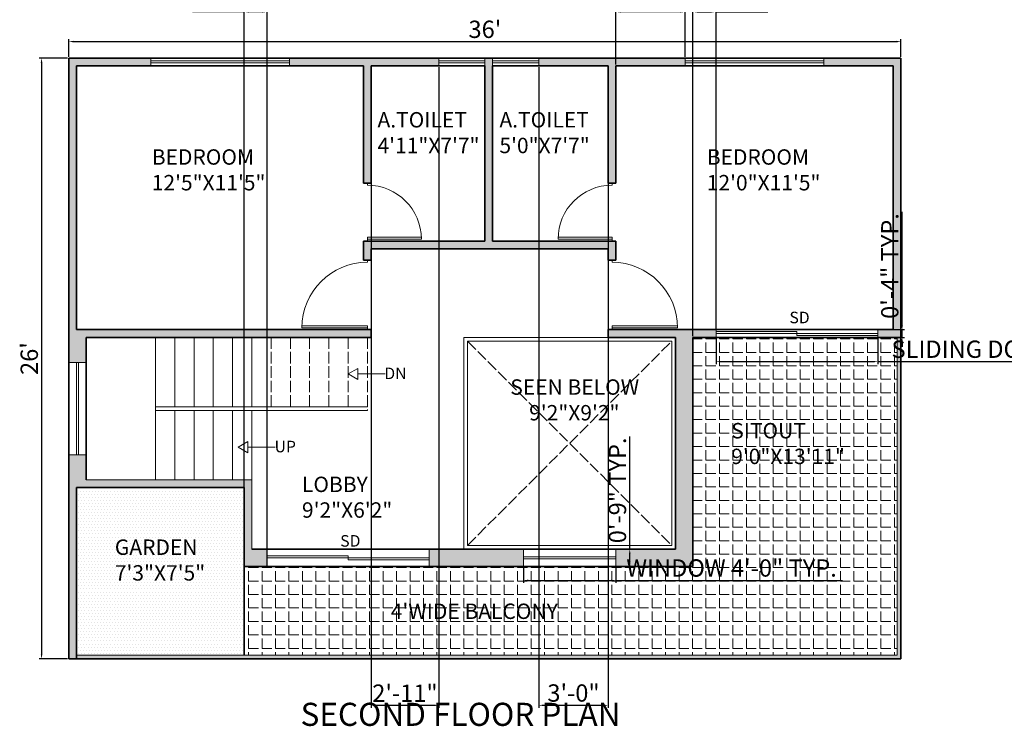
# Model space of a CAD drawing. Units: inches. Extents: x 1947 to 4744, y 610 to 1869.
# Tile 3 of 8: x 3688 to 4199, y 707 to 1074. Entities that reach past the tile are written whole.
import ezdxf

# ---------------------------------------------------------------- set-up
doc = ezdxf.new("R2010")
doc.units = ezdxf.units.IN
doc.linetypes.add('ACAD_ISO02W100', pattern=[15, 12, -3])
for name, color, linetype, lineweight in [('A-ANNO-DIMS', 2, 'Continuous', 18), ('A-ANNO-SYMB', 2, 'Continuous', 18), ('A-ANNO-TEXT', 7, 'Continuous', 18), ('A-ANNO-TITL', 7, 'Continuous', 35), ('A-AREA-IDEN', 7, 'Continuous', 18), ('A-DOOR', 3, 'Continuous', 18), ('A-FLOR-OPEN', 7, 'Continuous', 18), ('A-FLOR-OPEN-PROJ', 8, 'ACAD_ISO02W100', 13), ('A-FLOR-STRS', 7, 'Continuous', 18), ('A-FLOR-STRS-OVHD', 7, 'ACAD_ISO02W100', 13), ('A-GLAZ', 4, 'Continuous', 18), ('A-WALL', 7, 'Continuous', 35), ('A-WALL-PRHT', 7, 'Continuous', 18), ('L-PLNT-PATT', 3, 'Continuous', 13)]:
    doc.layers.add(name, color=color, linetype=linetype, lineweight=lineweight)
doc.layers.add('A-FLOR-PATT', color=251, linetype='Continuous', lineweight=13, true_color=0x636466)
doc.layers.add('A-WALL-PATT', color=18, linetype='Continuous', lineweight=13, true_color=0x000000)
doc.styles.get("Standard").update_dxf_attribs({"font": 'arial.ttf'})
doc.dimstyles.new('ISO-25', dxfattribs={"dimtxt": 9, "dimasz": 2.5, "dimexe": 1.25, "dimexo": 0.625, "dimtad": 1, "dimdec": 1, "dimlunit": 3, "dimtxsty": 'Standard', "dimcen": 2.5, "dimadec": 0, "dimazin": 0, "dimtfac": 1, "dimtdec": 1, "dimtmove": 0, "dimatfit": 3, "dimfxl": 1, "dimarcsym": 0})

# ---------------------------------------------------------------- blocks, each defined once
blk = doc.blocks.new('2')
for p, q in [((4319.45, 1679.18), (4319.45, 1713.18)), ((4320.45, 1679.18), (4320.45, 1713.18)), ((4318.45, 1679.18), (4320.45, 1679.18)), ((4353.45, 1679.18), (4354.45, 1679.18))]:
    blk.add_line(p, q)
at = {"ltscale": 0.5}
blk.add_arc((4319.45, 1679.18), 34, 0, 90, dxfattribs=at)
blk = doc.blocks.new('4')
for p, q in [((3808.6, 1693.11), (3808.6, 1721.11)), ((3809.6, 1693.11), (3809.6, 1721.11)), ((3807.6, 1693.11), (3809.6, 1693.11)), ((3836.6, 1693.11), (3837.6, 1693.11))]:
    blk.add_line(p, q)
at = {"ltscale": 0.5}
blk.add_arc((3808.6, 1693.11), 28, 0, 90, dxfattribs=at)
blk = doc.blocks.new('*D9')
at = {"layer": 'A-ANNO-DIMS', "color": 0, "lineweight": -2, "transparency": 16777216}
for p, q in [((3713.53, 1054.49), (3713.53, 1063.69)), ((4145.53, 1054.49), (4145.53, 1063.69)), ((3716.03, 1062.44), (4143.03, 1062.44))]:
    blk.add_line(p, q, dxfattribs=at)
at = {"layer": 'A-ANNO-DIMS', "color": 0, "transparency": 16777216}
for points in [[(3716.03, 1062.86), (3716.03, 1062.02), (3713.53, 1062.44)], [(4143.03, 1062.86), (4143.03, 1062.02), (4145.53, 1062.44)]]:
    blk.add_solid(points, dxfattribs=at)
at = {"layer": 'Defpoints', "color": 0, "transparency": 16777216}
for p in [(4145.53, 1062.44), (3713.53, 1053.87), (4145.53, 1053.87)]:
    blk.add_point(p, dxfattribs=at)
at = {"layer": 'A-ANNO-DIMS', "color": 0, "transparency": 16777216, "insert": (3929.53, 1067.66), "char_height": 9, "attachment_point": 5}
blk.add_mtext("36'", dxfattribs=at)
blk = doc.blocks.new('*D10')
at = {"layer": 'A-ANNO-DIMS', "color": 0, "lineweight": -2, "transparency": 16777216}
for p, q in [((3712.91, 1053.87), (3698.11, 1053.87)), ((3699.36, 1051.37), (3699.36, 744.37)), ((3712.91, 741.87), (3698.11, 741.87))]:
    blk.add_line(p, q, dxfattribs=at)
at = {"layer": 'A-ANNO-DIMS', "color": 0, "transparency": 16777216}
for points in [[(3698.94, 1051.37), (3699.77, 1051.37), (3699.36, 1053.87)], [(3698.94, 744.37), (3699.77, 744.37), (3699.36, 741.87)]]:
    blk.add_solid(points, dxfattribs=at)
at = {"layer": 'Defpoints', "color": 0, "transparency": 16777216}
for p in [(3713.53, 1053.87), (3699.36, 741.87), (3713.53, 741.87)]:
    blk.add_point(p, dxfattribs=at)
at = {"layer": 'A-ANNO-DIMS', "color": 0, "transparency": 16777216, "insert": (3694.14, 897.87), "char_height": 9, "attachment_point": 5, "rotation": 90}
blk.add_mtext("26'", dxfattribs=at)
blk = doc.blocks.new('WIN-72-4')
for p, q in [((0, 0), (0, 4)), ((72, 2.5), (0, 2.5)), ((72, 1.5), (0, 1.5)), ((72, 0), (72, 4))]:
    blk.add_line(p, q)
blk = doc.blocks.new('WIN-48-9')
for p, q in [((0, 0), (0, 9)), ((48, 0), (48, 9)), ((48, 5), (0, 5)), ((48, 4), (0, 4))]:
    blk.add_line(p, q)
blk = doc.blocks.new('WIN-24-4')
for p, q in [((0, 0), (0, 4)), ((24, 2.5), (0, 2.5)), ((24, 1.5), (0, 1.5)), ((24, 0), (24, 4))]:
    blk.add_line(p, q)
blk = doc.blocks.new('DOOR-SLIDE-84-9')
for p, q in [((0, 9), (0, 0)), ((42, 5.5), (0, 5.5)), ((42, 4.5), (42, 5.5)), ((84, 9), (84, 0)), ((0, 4.5), (84, 4.5)), ((42, 4.5), (42, 3.5)), ((42, 3.5), (84, 3.5))]:
    blk.add_line(p, q)
blk = doc.blocks.new('DOOR-SLIDE-84-4')
for p, q in [((0, 0), (0, 4)), ((42, 3), (0, 3)), ((0, 2), (84, 2)), ((42, 2), (42, 3)), ((42, 2), (42, 1)), ((42, 1), (84, 1)), ((84, 0), (84, 4))]:
    blk.add_line(p, q)
blk = doc.blocks.new('STAIR-DIRECTION')
blk.add_line((2.91, 14.18), (2.91, 0))
blk.add_lwpolyline([(2.91, 19.23), (0, 14.18), (5.83, 14.18)], close=True)
blk = doc.blocks.new('*D84')
at = {"layer": 'A-ANNO-DIMS', "color": 0, "lineweight": -2, "transparency": 16777216}
for p, q in [((3949.53, 789.24), (3949.53, 781.42)), ((3997.53, 789.24), (3997.53, 781.42)), ((3952.03, 782.67), (3995.03, 782.67)), ((3997.53, 782.67), (4115.17, 782.67))]:
    blk.add_line(p, q, dxfattribs=at)
at = {"layer": 'A-ANNO-DIMS', "color": 0, "transparency": 16777216}
for points in [[(3952.03, 783.08), (3952.03, 782.25), (3949.53, 782.67)], [(3995.03, 783.08), (3995.03, 782.25), (3997.53, 782.67)]]:
    blk.add_solid(points, dxfattribs=at)
at = {"layer": 'Defpoints', "color": 0, "transparency": 16777216}
for p in [(3949.53, 789.87), (3997.53, 789.87), (3997.53, 782.67)]:
    blk.add_point(p, dxfattribs=at)
at = {"layer": 'A-ANNO-DIMS', "color": 0, "transparency": 16777216, "insert": (4057.6, 787.95), "char_height": 9, "attachment_point": 5}
blk.add_mtext('WINDOW 4\'-0" TYP.', dxfattribs=at)
blk = doc.blocks.new('*D85')
at = {"layer": 'A-ANNO-DIMS', "color": 0, "lineweight": -2, "transparency": 16777216}
for p, q in [((4004.73, 798.87), (4004.73, 857.48)), ((3998.16, 798.87), (4005.98, 798.87)), ((4004.73, 792.37), (4004.73, 796.37)), ((3998.16, 789.87), (4005.98, 789.87))]:
    blk.add_line(p, q, dxfattribs=at)
at = {"layer": 'A-ANNO-DIMS', "color": 0, "transparency": 16777216}
for points in [[(4004.31, 796.37), (4005.15, 796.37), (4004.73, 798.87)], [(4004.31, 792.37), (4005.15, 792.37), (4004.73, 789.87)]]:
    blk.add_solid(points, dxfattribs=at)
at = {"layer": 'Defpoints', "color": 0, "transparency": 16777216}
for p in [(3997.53, 798.87), (4004.73, 798.87), (3997.53, 789.87)]:
    blk.add_point(p, dxfattribs=at)
at = {"layer": 'A-ANNO-DIMS', "color": 0, "transparency": 16777216, "insert": (3999.51, 829.42), "char_height": 9, "attachment_point": 5, "rotation": 90}
blk.add_mtext('0\'-9" TYP.', dxfattribs=at)
blk = doc.blocks.new('*D92')
at = {"layer": 'A-ANNO-DIMS', "color": 0, "lineweight": -2, "transparency": 16777216}
for p, q in [((4049.53, 908.24), (4049.53, 895.02)), ((4133.53, 908.24), (4133.53, 895.02)), ((4052.03, 896.27), (4131.03, 896.27)), ((4133.53, 896.27), (4287.11, 896.27))]:
    blk.add_line(p, q, dxfattribs=at)
at = {"layer": 'A-ANNO-DIMS', "color": 0, "transparency": 16777216}
for points in [[(4052.03, 896.68), (4052.03, 895.85), (4049.53, 896.27)], [(4131.03, 896.68), (4131.03, 895.85), (4133.53, 896.27)]]:
    blk.add_solid(points, dxfattribs=at)
at = {"layer": 'Defpoints', "color": 0, "transparency": 16777216}
for p in [(4049.53, 908.87), (4133.53, 908.87), (4133.53, 896.27)]:
    blk.add_point(p, dxfattribs=at)
at = {"layer": 'A-ANNO-DIMS', "color": 0, "transparency": 16777216, "insert": (4211.57, 901.55), "char_height": 9, "attachment_point": 5}
blk.add_mtext('SLIDING DOOR 7\'-0" TYP.', dxfattribs=at)
blk = doc.blocks.new('*D93')
at = {"layer": 'A-ANNO-DIMS', "color": 0, "lineweight": -2, "transparency": 16777216}
for p, q in [((4146.13, 915.37), (4146.13, 973.98)), ((4134.16, 912.87), (4147.38, 912.87)), ((4146.13, 908.87), (4146.13, 912.87)), ((4134.16, 908.87), (4147.38, 908.87)), ((4146.13, 906.37), (4146.13, 903.87))]:
    blk.add_line(p, q, dxfattribs=at)
at = {"layer": 'A-ANNO-DIMS', "color": 0, "transparency": 16777216}
for points in [[(4145.71, 915.37), (4146.55, 915.37), (4146.13, 912.87)], [(4145.71, 906.37), (4146.55, 906.37), (4146.13, 908.87)]]:
    blk.add_solid(points, dxfattribs=at)
at = {"layer": 'Defpoints', "color": 0, "transparency": 16777216}
for p in [(4133.53, 912.87), (4146.13, 912.87), (4133.53, 908.87)]:
    blk.add_point(p, dxfattribs=at)
at = {"layer": 'A-ANNO-DIMS', "color": 0, "transparency": 16777216, "insert": (4140.91, 945.92), "char_height": 9, "attachment_point": 5, "rotation": 90}
blk.add_mtext('0\'-4" TYP.', dxfattribs=at)
blk = doc.blocks.new('*D110')
at = {"layer": 'A-ANNO-DIMS', "color": 0, "lineweight": -2, "transparency": 16777216}
for p, q in [((3997.53, 1050.49), (3997.53, 1079.17)), ((4033.53, 1054.49), (4033.53, 1079.17)), ((4031.03, 1077.92), (4000.03, 1077.92))]:
    blk.add_line(p, q, dxfattribs=at)
at = {"layer": 'A-ANNO-DIMS', "color": 0, "transparency": 16777216}
for points in [[(4000.03, 1078.33), (4000.03, 1077.5), (3997.53, 1077.92)], [(4031.03, 1078.33), (4031.03, 1077.5), (4033.53, 1077.92)]]:
    blk.add_solid(points, dxfattribs=at)
at = {"layer": 'Defpoints', "color": 0, "transparency": 16777216}
for p in [(3997.53, 1077.92), (4033.53, 1053.87), (3997.53, 1049.87)]:
    blk.add_point(p, dxfattribs=at)
at = {"layer": 'A-ANNO-DIMS', "color": 0, "transparency": 16777216, "insert": (4015.53, 1083.14), "char_height": 9, "attachment_point": 5}
blk.add_mtext('3\'-0"', dxfattribs=at)
blk = doc.blocks.new('*D113')
at = {"layer": 'A-ANNO-DIMS', "color": 0, "lineweight": -2, "transparency": 16777216}
for p, q in [((4037.53, 909.49), (4037.53, 1079.17)), ((4049.53, 913.49), (4049.53, 1079.17)), ((4040.03, 1077.92), (4047.03, 1077.92)), ((4049.53, 1077.92), (4076.36, 1077.92))]:
    blk.add_line(p, q, dxfattribs=at)
at = {"layer": 'A-ANNO-DIMS', "color": 0, "transparency": 16777216}
for points in [[(4040.03, 1078.33), (4040.03, 1077.5), (4037.53, 1077.92)], [(4047.03, 1078.33), (4047.03, 1077.5), (4049.53, 1077.92)]]:
    blk.add_solid(points, dxfattribs=at)
at = {"layer": 'Defpoints', "color": 0, "transparency": 16777216}
for p in [(4049.53, 1077.92), (4049.53, 912.87), (4037.53, 908.87)]:
    blk.add_point(p, dxfattribs=at)
at = {"layer": 'A-ANNO-DIMS', "color": 0, "transparency": 16777216, "insert": (4064.19, 1083.14), "char_height": 9, "attachment_point": 5}
blk.add_mtext('1\'-0"', dxfattribs=at)
blk = doc.blocks.new('*D114')
at = {"layer": 'A-ANNO-DIMS', "color": 0, "lineweight": -2, "transparency": 16777216}
for p, q in [((3804.53, 790.49), (3804.53, 1079.17)), ((3816.53, 790.49), (3816.53, 1079.17)), ((3804.53, 1077.92), (3777.7, 1077.92)), ((3814.03, 1077.92), (3807.03, 1077.92))]:
    blk.add_line(p, q, dxfattribs=at)
at = {"layer": 'A-ANNO-DIMS', "color": 0, "transparency": 16777216}
for points in [[(3807.03, 1078.33), (3807.03, 1077.5), (3804.53, 1077.92)], [(3814.03, 1078.33), (3814.03, 1077.5), (3816.53, 1077.92)]]:
    blk.add_solid(points, dxfattribs=at)
at = {"layer": 'Defpoints', "color": 0, "transparency": 16777216}
for p in [(3804.53, 1077.92), (3804.53, 789.87), (3816.53, 789.87)]:
    blk.add_point(p, dxfattribs=at)
at = {"layer": 'A-ANNO-DIMS', "color": 0, "transparency": 16777216, "insert": (3789.87, 1083.14), "char_height": 9, "attachment_point": 5}
blk.add_mtext('1\'-0"', dxfattribs=at)
blk = doc.blocks.new('*D117')
at = {"layer": 'A-ANNO-DIMS', "color": 0, "lineweight": -2, "transparency": 16777216}
for p, q in [((3870.53, 1049.24), (3870.53, 716.57)), ((3905.53, 1049.24), (3905.53, 716.57)), ((3873.03, 717.82), (3903.03, 717.82))]:
    blk.add_line(p, q, dxfattribs=at)
at = {"layer": 'A-ANNO-DIMS', "color": 0, "transparency": 16777216}
for points in [[(3873.03, 718.23), (3873.03, 717.4), (3870.53, 717.82)], [(3903.03, 718.23), (3903.03, 717.4), (3905.53, 717.82)]]:
    blk.add_solid(points, dxfattribs=at)
at = {"layer": 'Defpoints', "color": 0, "transparency": 16777216}
for p in [(3870.53, 1049.87), (3905.53, 1049.87), (3905.53, 717.82)]:
    blk.add_point(p, dxfattribs=at)
at = {"layer": 'A-ANNO-DIMS', "color": 0, "transparency": 16777216, "insert": (3888.03, 722.96), "char_height": 9, "attachment_point": 5}
blk.add_mtext('2\'-11"', dxfattribs=at)
blk = doc.blocks.new('*D118')
at = {"layer": 'A-ANNO-DIMS', "color": 0, "lineweight": -2, "transparency": 16777216}
for p, q in [((3957.53, 1049.24), (3957.53, 716.57)), ((3993.53, 1049.24), (3993.53, 716.57)), ((3960.03, 717.82), (3991.03, 717.82))]:
    blk.add_line(p, q, dxfattribs=at)
at = {"layer": 'A-ANNO-DIMS', "color": 0, "transparency": 16777216}
for points in [[(3960.03, 718.23), (3960.03, 717.4), (3957.53, 717.82)], [(3991.03, 718.23), (3991.03, 717.4), (3993.53, 717.82)]]:
    blk.add_solid(points, dxfattribs=at)
at = {"layer": 'Defpoints', "color": 0, "transparency": 16777216}
for p in [(3957.53, 1049.87), (3993.53, 1049.87), (3993.53, 717.82)]:
    blk.add_point(p, dxfattribs=at)
at = {"layer": 'A-ANNO-DIMS', "color": 0, "transparency": 16777216, "insert": (3975.53, 723.04), "char_height": 9, "attachment_point": 5}
blk.add_mtext('3\'-0"', dxfattribs=at)

msp = doc.modelspace()

# ---------------------------------------------------------------- hatches: boundary and pattern name
at = {"layer": 'A-FLOR-PATT'}
h = msp.add_hatch(dxfattribs=at)
h.set_pattern_fill('ANGLE', color=256)
h.set_pattern_definition([(0, (0, 0), (0, 6.985), [5.08, -1.905]), (90, (0, 0), (-6.985, 4e-16), [5.08, -1.905])])
h.paths.add_polyline_path([(4143.53, 743.87), (4143.53, 908.87), (4037.53, 908.87), (4037.53, 789.87), (3804.53, 789.87), (3804.53, 743.87)])
h.paths.add_polyline_path([(3878.47, 758.1), (3981.39, 758.1), (3981.39, 775.18), (3878.47, 775.18)], flags=24)
h.paths.add_polyline_path([(4054.68, 838.52), (4116.82, 838.52), (4116.82, 868.94), (4054.68, 868.94)], flags=24)
at = {"layer": 'A-WALL-PATT'}
h = msp.add_hatch(color=256, dxfattribs=at)
h.dxf.hatch_style = 1
h.paths.add_polyline_path([(3933.53, 1049.87), (3933.53, 1053.87), (3929.53, 1053.87), (3929.53, 1049.87), (3929.53, 958.87), (3866.53, 958.87), (3866.53, 948.87), (3870.53, 948.87), (3870.53, 954.87), (3993.53, 954.87), (3993.53, 948.87), (3997.53, 948.87), (3997.53, 958.87), (3933.53, 958.87)])
h.paths.add_polyline_path([(4033.53, 1053.87), (3957.53, 1053.87), (3957.53, 1049.87), (3993.53, 1049.87), (3993.53, 988.87), (3997.53, 988.87), (3997.53, 1049.87), (4033.53, 1049.87)])
h.paths.add_polyline_path([(3905.53, 1053.87), (3828.03, 1053.87), (3828.03, 1049.87), (3866.53, 1049.87), (3866.53, 988.87), (3870.53, 988.87), (3870.53, 1049.87), (3905.53, 1049.87)])
h.paths.add_polyline_path([(4145.53, 1053.87), (4105.53, 1053.87), (4105.53, 1049.87), (4141.53, 1049.87), (4141.53, 912.87), (4133.53, 912.87), (4133.53, 908.87), (4145.53, 908.87)])
h.paths.add_polyline_path([(4037.53, 908.87), (4049.53, 908.87), (4049.53, 912.87), (3993.53, 912.87), (3993.53, 908.87), (4028.53, 908.87), (4028.53, 798.87), (3997.53, 798.87), (3997.53, 789.87), (4037.53, 789.87)])
h.paths.add_polyline_path([(3949.53, 798.87), (3900.53, 798.87), (3900.53, 789.87), (3949.53, 789.87)], flags=17)
h.paths.add_polyline_path([(3816.53, 798.87), (3808.53, 798.87), (3808.53, 834.87), (3722.53, 834.87), (3722.53, 847.87), (3713.53, 847.87), (3713.53, 741.87), (3717.53, 741.87), (3717.53, 830.87), (3804.53, 830.87), (3804.53, 789.87), (3816.53, 789.87)])
h.paths.add_polyline_path([(3722.53, 908.87), (3870.53, 908.87), (3870.53, 912.87), (3717.53, 912.87), (3717.53, 1049.87), (3756.03, 1049.87), (3756.03, 1053.87), (3713.53, 1053.87), (3713.53, 895.87), (3722.53, 895.87)])
h.paths.add_polyline_path([(4145.53, 908.87), (4143.53, 908.87), (4143.53, 743.87), (3717.53, 743.87), (3717.53, 741.87), (4145.53, 741.87)])
at = {"layer": 'L-PLNT-PATT'}
h = msp.add_hatch(dxfattribs=at)
h.set_pattern_fill('DOTS', color=256)
h.set_pattern_definition([(0, (0, -6.0122), (0.79375, 1.5875), [0, -1.5875])])
h.paths.add_polyline_path([(3804.53, 743.87), (3804.53, 830.87), (3717.53, 830.87), (3717.53, 743.87)])
h.paths.add_polyline_path([(3734.98, 778.03), (3788.22, 778.03), (3788.22, 808.45), (3734.98, 808.45)], flags=24)

# ---------------------------------------------------------------- linework, layer by layer
at = {"layer": 'A-FLOR-OPEN'}
for points in [[(4028.53, 798.87), (3918.53, 798.87), (3918.53, 908.87), (4028.53, 908.87)], [(4026.53, 800.87), (3920.53, 800.87), (3920.53, 906.87), (4026.53, 906.87)]]:
    msp.add_lwpolyline(points, close=True, dxfattribs=at)
at = {"layer": 'A-FLOR-OPEN-PROJ', "ltscale": 0.5}
for p, q in [((3920.53, 906.87), (4026.53, 800.87)), ((3920.53, 800.87), (4026.53, 906.87))]:
    msp.add_line(p, q, dxfattribs=at)
at = {"layer": 'A-FLOR-STRS'}
for p, q in [((3758.53, 908.87), (3758.53, 834.87)), ((3768.53, 908.87), (3768.53, 872.87)), ((3778.53, 908.87), (3778.53, 872.87)), ((3788.53, 908.87), (3788.53, 872.87)), ((3798.53, 908.87), (3798.53, 872.87)), ((3808.53, 908.87), (3808.53, 872.87)), ((3868.53, 872.87), (3758.53, 872.87)), ((3758.53, 870.87), (3868.53, 870.87)), ((3768.53, 870.87), (3768.53, 834.87)), ((3778.53, 870.87), (3778.53, 834.87)), ((3788.53, 870.87), (3788.53, 834.87)), ((3798.53, 870.87), (3798.53, 834.87)), ((3808.53, 870.87), (3808.53, 798.87)), ((3722.53, 834.87), (3808.53, 834.87))]:
    msp.add_line(p, q, dxfattribs=at)
at = {"layer": 'A-FLOR-STRS-OVHD', "ltscale": 0.5}
for p, q in [((3818.53, 908.87), (3818.53, 872.87)), ((3828.53, 908.87), (3828.53, 872.87)), ((3838.53, 908.87), (3838.53, 872.87)), ((3848.53, 908.87), (3848.53, 872.87)), ((3858.53, 908.87), (3858.53, 872.87)), ((3868.53, 908.87), (3868.53, 870.87))]:
    msp.add_line(p, q, dxfattribs=at)
at = {"layer": 'A-WALL'}
for p, q in [((4145.53, 1053.87), (3713.53, 1053.87)), ((3713.53, 1053.87), (3713.53, 741.87)), ((4145.53, 741.87), (4145.53, 1053.87)), ((3717.53, 1049.87), (3717.53, 912.87)), ((3866.53, 1049.87), (3717.53, 1049.87)), ((3866.53, 1049.87), (3866.53, 988.87)), ((3870.53, 1049.87), (3870.53, 988.87)), ((3929.53, 1049.87), (3870.53, 1049.87)), ((3929.53, 958.87), (3929.53, 1049.87)), ((3933.53, 958.87), (3933.53, 1049.87)), ((3993.53, 1049.87), (3933.53, 1049.87)), ((3993.53, 988.87), (3993.53, 1049.87)), ((4141.53, 1049.87), (3997.53, 1049.87)), ((3997.53, 988.87), (3997.53, 1049.87)), ((4141.53, 912.87), (4141.53, 1049.87)), ((3870.53, 988.87), (3866.53, 988.87)), ((3997.53, 988.87), (3993.53, 988.87)), ((3929.53, 958.87), (3866.53, 958.87)), ((3866.53, 958.87), (3866.53, 948.87)), ((3997.53, 958.87), (3933.53, 958.87)), ((3997.53, 948.87), (3997.53, 958.87)), ((3993.53, 954.87), (3870.53, 954.87)), ((3870.53, 954.87), (3870.53, 948.87)), ((3993.53, 948.87), (3993.53, 954.87)), ((3870.53, 948.87), (3866.53, 948.87)), ((3993.53, 948.87), (3997.53, 948.87)), ((3870.53, 912.87), (3717.53, 912.87)), ((3870.53, 912.87), (3870.53, 908.87)), ((3993.53, 912.87), (4141.53, 912.87)), ((3993.53, 908.87), (3993.53, 912.87)), ((3870.53, 908.87), (3722.53, 908.87)), ((3722.53, 908.87), (3722.53, 834.87)), ((3993.53, 908.87), (4028.53, 908.87)), ((4028.53, 798.87), (4028.53, 908.87)), ((4037.53, 789.87), (4037.53, 908.87)), ((4037.53, 908.87), (4145.53, 908.87)), ((3717.53, 830.87), (3717.53, 741.87)), ((3717.53, 830.87), (3804.53, 830.87)), ((3804.53, 830.87), (3804.53, 743.87)), ((3808.53, 798.87), (4028.53, 798.87)), ((3804.53, 789.87), (4037.53, 789.87)), ((3713.53, 741.87), (4145.53, 741.87))]:
    msp.add_line(p, q, dxfattribs=at)
at = {"layer": 'A-WALL-PRHT'}
for p, q in [((4143.53, 743.87), (4143.53, 908.87)), ((3717.53, 743.87), (4143.53, 743.87))]:
    msp.add_line(p, q, dxfattribs=at)

# ---------------------------------------------------------------- block references
at = {"layer": 'A-ANNO-SYMB'}
for p, rotation in [((3877.73, 886.95), 89.99999999999952), ((3820.7, 848.95), 90.00000000000047)]:
    msp.add_blockref('STAIR-DIRECTION', p, dxfattribs=dict(at, rotation=rotation))
at = {"layer": 'A-DOOR', "xscale": -1, "rotation": 270}
for name, p in [('4', (2175.42, -2848.73)), ('2', (2316.35, -3405.59))]:
    msp.add_blockref(name, p, dxfattribs=at)
at = {"layer": 'A-DOOR', "rotation": 90.00000000000003}
for name, p in [('4', (5688.64, -2848.73)), ('2', (5547.71, -3405.59))]:
    msp.add_blockref(name, p, dxfattribs=at)
at = {"layer": 'A-DOOR'}
for name, p in [('DOOR-SLIDE-84-4', (4049.53, 908.87)), ('DOOR-SLIDE-84-9', (3816.53, 789.87))]:
    msp.add_blockref(name, p, dxfattribs=at)
at = {"layer": 'A-GLAZ'}
for name, p in [('WIN-72-4', (3756.03, 1049.87)), ('WIN-24-4', (3905.53, 1049.87)), ('WIN-72-4', (4033.53, 1049.87)), ('WIN-48-9', (3949.53, 789.87))]:
    msp.add_blockref(name, p, dxfattribs=at)
for name, p, rotation in [('WIN-24-4', (3957.53, 1053.87), 180), ('WIN-48-9', (3722.53, 847.87), 89.99999999999928)]:
    msp.add_blockref(name, p, dxfattribs=dict(at, rotation=rotation))

# ---------------------------------------------------------------- texts
at = {"layer": 'A-ANNO-TEXT', "char_height": 6, "attachment_point": 1}
for s, insert in [('{\\fTimes New Roman|b0|i0|c0|p18;SD}', (4087.63, 922.19)), ('{\\fTimes New Roman|b0|i0|c0|p18;DN}', (3877.31, 893.18)), ('{\\fTimes New Roman|b0|i0|c0|p18;UP}', (3820.33, 855.18)), ('{\\fTimes New Roman|b0|i0|c0|p18;SD}', (3854.42, 806.2))]:
    msp.add_mtext_dynamic_manual_height_columns(s, width=158.3328, gutter_width=12.5, heights=[0], dxfattribs=dict(at, insert=insert))
at = {"layer": 'A-ANNO-TITL', "insert": (3833.83, 719.13), "char_height": 12, "attachment_point": 1}
msp.add_mtext_dynamic_manual_height_columns('{\\fTimes New Roman|b0|i0|c0|p18;SECOND FLOOR PLAN}', width=253.4596, gutter_width=12.5, heights=[0], dxfattribs=at)
at = {"layer": 'A-AREA-IDEN', "char_height": 8, "attachment_point": 1}
for s, width, insert in [('{\\fTimes New Roman|b0|i0|c0|p18;A.TOILET\\P4\'11"X7\'7"}', 64.3566, (3873.77, 1025.84)), ('{\\fTimes New Roman|b0|i0|c0|p18;A.TOILET\\P5\'0"X7\'7"}', 64.3566, (3937.07, 1025.84)), ('{\\fTimes New Roman|b0|i0|c0|p18;BEDROOM\\P12\'5"X11\'5"}', 64.3566, (3756.58, 1006.52)), ('{\\fTimes New Roman|b0|i0|c0|p18;BEDROOM\\P12\'0"X11\'5"}', 64.3566, (4044.73, 1006.52)), ('{\\fTimes New Roman|b0|i0|c0|p18;SEEN BELOW\\P    9\'2"X9\'2"}', 135.7043, (3942.72, 887.07)), ('{\\fTimes New Roman|b0|i0|c0|p18;SITOUT\\P9\'0"X13\'11"}', 64.3566, (4057.42, 864.41)), ('{\\fTimes New Roman|b0|i0|c0|p18;LOBBY\\P9\'2"X6\'2"}', 64.3566, (3834.56, 836.55)), ('{\\fTimes New Roman|b0|i0|c0|p18;GARDEN\\P7\'3"X7\'5"}', 64.3566, (3737.41, 803.92)), ("{\\fTimes New Roman|b0|i0|c0|p18;4'WIDE BALCONY}", 158.3328, (3880.66, 770.65))]:
    msp.add_mtext_dynamic_manual_height_columns(s, width=width, gutter_width=12.5, heights=[0], dxfattribs=dict(at, insert=insert))

# ---------------------------------------------------------------- dimensions: what is measured, and where the dimension line sits
at = {"layer": 'A-ANNO-DIMS'}
for base, p1, p2, override, picture, middle in [((3804.53, 1077.92), (3816.53, 789.87), (3804.53, 789.87), {"dimdec": 1, "dimlfac": 1, "dimrnd": 0, "dimzin": 1, "dimdsep": 46, "dimlunit": 4, "dimfrac": 2}, '*D114', (3789.87, 1083.14)), ((3997.53, 1077.92), (4033.53, 1053.87), (3997.53, 1049.87), {"dimdec": 1, "dimlfac": 1, "dimrnd": 0, "dimzin": 1, "dimdsep": 46, "dimlunit": 4, "dimfrac": 2}, '*D110', (4015.53, 1083.14)), ((4049.53, 1077.92), (4037.53, 908.87), (4049.53, 912.87), {"dimdec": 1, "dimlfac": 1, "dimrnd": 0, "dimzin": 1, "dimdsep": 46, "dimlunit": 4, "dimfrac": 2}, '*D113', (4064.19, 1083.14)), ((4145.53, 1062.44), (3713.53, 1053.87), (4145.53, 1053.87), {"dimclrd": 0, "dimclre": 0, "dimclrt": 0}, '*D9', (3929.53, 1067.66)), ((3905.53, 717.82), (3870.53, 1049.87), (3905.53, 1049.87), {"dimdec": 1, "dimlfac": 1, "dimrnd": 0, "dimzin": 1, "dimdsep": 46, "dimlunit": 4, "dimfrac": 2}, '*D117', (3888.03, 722.96)), ((3993.53, 717.82), (3957.53, 1049.87), (3993.53, 1049.87), {"dimdec": 1, "dimlfac": 1, "dimrnd": 0, "dimzin": 1, "dimdsep": 46, "dimlunit": 4, "dimfrac": 2}, '*D118', (3975.53, 723.04))]:
    dim = msp.add_linear_dim(base=base, p1=p1, p2=p2, dimstyle='ISO-25', override=override, dxfattribs=at)
    dim.commit()
    dim.dimension.update_dxf_attribs({"geometry": picture, "text_midpoint": middle})
dim = msp.add_linear_dim(base=(3699.36, 741.87), p1=(3713.53, 1053.87), p2=(3713.53, 741.87), angle=90, dimstyle='ISO-25', override={"dimclrd": 0, "dimclre": 0, "dimclrt": 0}, dxfattribs=at)
dim.commit()
dim.dimension.update_dxf_attribs({"geometry": '*D10', "text_midpoint": (3694.14, 897.87)})
for base, p1, p2, picture, middle in [((4146.13, 912.87), (4133.53, 908.87), (4133.53, 912.87), '*D93', (4140.91, 945.92)), ((4004.73, 798.87), (3997.53, 789.87), (3997.53, 798.87), '*D85', (3999.51, 829.42))]:
    dim = msp.add_linear_dim(base=base, p1=p1, p2=p2, angle=90, text='<> TYP.', dimstyle='ISO-25', override={"dimdec": 1, "dimlfac": 1, "dimrnd": 0, "dimzin": 1, "dimdsep": 46, "dimlunit": 4, "dimfrac": 2}, dxfattribs=at)
    dim.commit()
    dim.dimension.update_dxf_attribs({"geometry": picture, "text_midpoint": middle})
for base, p1, p2, text, picture, middle in [((4133.53, 896.27), (4049.53, 908.87), (4133.53, 908.87), 'SLIDING DOOR <> TYP.', '*D92', (4211.57, 901.55)), ((3997.53, 782.67), (3949.53, 789.87), (3997.53, 789.87), 'WINDOW <> TYP.', '*D84', (4057.6, 787.95))]:
    dim = msp.add_linear_dim(base=base, p1=p1, p2=p2, text=text, dimstyle='ISO-25', override={"dimdec": 1, "dimlfac": 1, "dimrnd": 0, "dimzin": 1, "dimdsep": 46, "dimlunit": 4, "dimfrac": 2}, dxfattribs=at)
    dim.commit()
    dim.dimension.update_dxf_attribs({"geometry": picture, "text_midpoint": middle})

doc.saveas('drawing.dxf')
